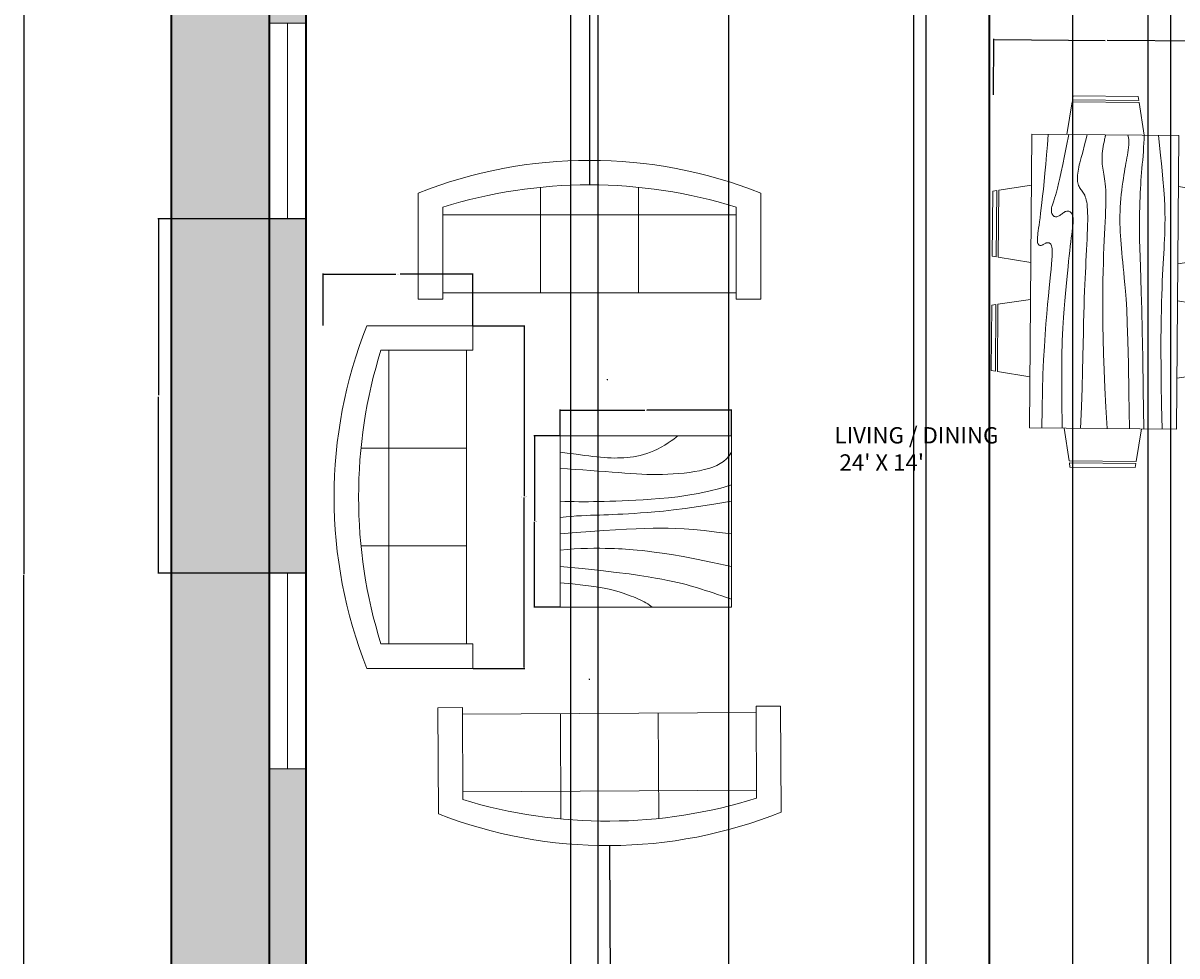
# Model space of a CAD drawing. Units: inches. Extents: x -7 to 546, y -27 to 766.
# Tile 5 of 9: x -7 to 276, y 276 to 505. Entities that reach past the tile are written whole.
import ezdxf

# ---------------------------------------------------------------- set-up
doc = ezdxf.new("R2010")
doc.units = ezdxf.units.IN
doc.header["$MEASUREMENT"] = 0
for name, color, linetype, lineweight in [('A-ANNO-DIMS', 2, 'Continuous', 18), ('A-AREA-IDEN', 7, 'Continuous', 18), ('A-WALL', 7, 'Continuous', 35), ('C-PROP', 7, 'Continuous', 35), ('furniture', 220, 'Continuous', 18), ('window', 30, 'Continuous', 20)]:
    doc.layers.add(name, color=color, linetype=linetype, lineweight=lineweight)
doc.layers.add('A-WALL-PATT', color=251, linetype='Continuous', lineweight=13, true_color=0x636466)
doc.layers.add('L-PLNT-PATT', color=85, linetype='Continuous', lineweight=13, true_color=0x58ba48)
doc.styles.get("Standard").update_dxf_attribs({"font": 'arial.ttf'})
doc.dimstyles.get("Standard").update_dxf_attribs({"dimtxt": 0.18, "dimasz": 0.18, "dimexe": 0.18, "dimexo": 0.0625, "dimgap": 0.09, "dimtad": 0, "dimtih": 1, "dimtoh": 1, "dimdec": 4, "dimzin": 0, "dimdsep": 46, "dimtxsty": 'Standard', "dimcen": 0.09, "dimadec": 0, "dimazin": 0, "dimtfac": 1, "dimtdec": 4, "dimtofl": 0, "dimtmove": 0, "dimatfit": 3, "dimfxl": 1, "dimtolj": 1, "dimtzin": 0, "dimarcsym": 0})

# ---------------------------------------------------------------- blocks, each defined once
blk = doc.blocks.new('Dining Set - 36 x 72 in.')
for p, q in [((-22.2343, 26.00059), (-23.4847, 17.99762)), ((-22.2304, 26), (-5.7608, 26)), ((-22, 27.5), (-22.1562, 26.50042)), ((-5.8416, 26.5), (-22.1534, 26.5)), ((-22, 27.5), (-6, 27.5)), ((-5.8437, 26.49966), (-6, 27.5)), ((-4.5152, 17.99762), (-5.7655, 25.99926)), ((5.7657, 26.00059), (4.5153, 17.99762)), ((5.7696, 26), (22.2392, 26)), ((6, 27.5), (5.8438, 26.50042)), ((22.1584, 26.5), (5.8466, 26.5)), ((6, 27.5), (22, 27.5)), ((22.1563, 26.49966), (22, 27.5)), ((23.4848, 17.99762), (22.2345, 25.99926)), ((36, 18), (-36, 18)), ((-36, 18), (-36, -18)), ((36, -18), (36, 18)), ((-44.0006, 8.23428), (-35.9976, 9.48474)), ((44.0006, 8.23428), (35.9976, 9.48474)), ((-45.5, 8), (-44.5004, 8.15617)), ((-45.5, 8), (-45.5, -8)), ((-44.5, -8.15843), (-44.5, 8.15338)), ((-44, 8.23041), (-44, -8.23915)), ((44, 8.23041), (44, -8.23915)), ((44.5, -8.15843), (44.5, 8.15338)), ((45.5, 8), (44.5005, 8.15617)), ((45.5, 8), (45.5, -8)), ((-44.4997, -8.15631), (-45.5, -8)), ((-35.9976, -9.48476), (-43.9993, -8.2345)), ((35.9976, -9.48476), (43.9993, -8.2345)), ((44.4997, -8.15631), (45.5, -8)), ((-36, -18), (36, -18)), ((-22.2343, -26.0006), (-23.4847, -17.99762)), ((-4.5152, -17.99762), (-5.7655, -25.99928)), ((5.7657, -26.0006), (4.5153, -17.99762)), ((23.4848, -17.99762), (22.2345, -25.99928)), ((-22.2304, -26), (-5.7608, -26)), ((-22, -27.5), (-22.1562, -26.50044)), ((-5.8416, -26.5), (-22.1534, -26.5)), ((-22, -27.5), (-6, -27.5)), ((-5.8437, -26.49967), (-6, -27.5)), ((5.7696, -26), (22.2392, -26)), ((6, -27.5), (5.8438, -26.50044)), ((22.1584, -26.5), (5.8466, -26.5)), ((6, -27.5), (22, -27.5)), ((22.1563, -26.49967), (22, -27.5))]:
    blk.add_line(p, q)
for points in [[(-36, 15), (-31.1772, 14.97754), (-26.8079, 14.91406), (-22.8538, 14.81543), (-19.276, 14.6875), (-16.0362, 14.53613), (-13.0957, 14.36718), (-10.4159, 14.18652), (-7.9583, 14), (-5.6904, 13.81315), (-3.6035, 13.63021), (-1.6954, 13.45508), (0.0365, 13.29166), (1.5945, 13.14388), (2.9811, 13.01562), (4.1988, 12.9108), (5.25, 12.83333), (6.1393, 12.78613), (6.8802, 12.76823), (7.4883, 12.77767), (7.9792, 12.8125), (8.3685, 12.87077), (8.6719, 12.95052), (8.9049, 13.0498), (9.0833, 13.16666), (9.2205, 13.29899), (9.3216, 13.44401), (9.3895, 13.59879), (9.4271, 13.76041), (9.4373, 13.92594), (9.4232, 14.09245), (9.3875, 14.257), (9.3333, 14.41666), (9.2638, 14.56917), (9.1836, 14.71484), (9.0975, 14.85465), (9.0104, 14.98958), (8.9272, 15.1206), (8.8529, 15.2487), (8.7922, 15.37483), (8.75, 15.5), (8.7305, 15.62467), (8.7344, 15.74739), (8.7617, 15.86621), (8.8125, 15.97916), (8.8867, 16.08431), (8.9844, 16.17968), (9.1055, 16.26334), (9.25, 16.33333), (9.4189, 16.38802), (9.6172, 16.42708), (9.8506, 16.45052), (10.125, 16.45833), (10.4463, 16.45052), (10.8203, 16.42708), (11.2529, 16.38802), (11.75, 16.33333), (12.3184, 16.26318), (12.9694, 16.17838), (13.7151, 16.07991), (14.5677, 15.96875), (15.5395, 15.84586), (16.6426, 15.71224), (17.8893, 15.56884), (19.2917, 15.41666), (20.859, 15.25667), (22.5879, 15.08984), (24.4721, 14.91715), (26.5052, 14.73958), (28.6809, 14.5581), (30.9929, 14.3737), (33.4347, 14.18733), (36, 14)], [(-36, 10), (-28.9766, 10.14274), (-23.1725, 10.20442), (-18.4241, 10.19775), (-14.5677, 10.13541), (-11.4399, 10.03011), (-8.877, 9.89453), (-6.7154, 9.74137), (-4.7917, 9.58333), (-2.9698, 9.43082), (-1.2246, 9.28515), (0.4415, 9.14534), (2.026, 9.01041), (3.5266, 8.87939), (4.9408, 8.7513), (6.266, 8.62516), (7.5, 8.5), (8.6411, 8.37549), (9.6914, 8.2539), (10.6538, 8.13818), (11.5312, 8.03125), (12.3267, 7.93603), (13.043, 7.85547), (13.6831, 7.79248), (14.25, 7.75), (14.7471, 7.7303), (15.1797, 7.73307), (15.5537, 7.75732), (15.875, 7.80208), (16.1494, 7.86637), (16.3828, 7.94922), (16.5811, 8.04964), (16.75, 8.16666), (16.8944, 8.29915), (17.0143, 8.44531), (17.1089, 8.60319), (17.1771, 8.77083), (17.218, 8.94629), (17.2305, 9.1276), (17.2137, 9.31282), (17.1667, 9.5), (17.0895, 9.6875), (16.987, 9.875), (16.8649, 10.0625), (16.7292, 10.25), (16.5856, 10.4375), (16.4401, 10.625), (16.2985, 10.8125), (16.1667, 11), (16.05, 11.18733), (15.9518, 11.3737), (15.8752, 11.5581), (15.8229, 11.73958), (15.798, 11.91715), (15.8034, 12.08984), (15.842, 12.25667), (15.9167, 12.41666), (16.0295, 12.56836), (16.1784, 12.70833), (16.3605, 12.83268), (16.5729, 12.9375), (16.8127, 13.01888), (17.0768, 13.07291), (17.3625, 13.0957), (17.6667, 13.08333), (17.9894, 13.03312), (18.3418, 12.94726), (18.7382, 12.82918), (19.1927, 12.68229), (19.7195, 12.51001), (20.3327, 12.31575), (21.0465, 12.10294), (21.875, 11.875), (22.8357, 11.63354), (23.959, 11.37304), (25.2786, 11.08618), (26.8282, 10.76562), (28.6414, 10.40405), (30.752, 9.99414), (33.1936, 9.52856), (36, 9)], [(-36, 5.5), (-30.7157, 5.3348), (-26.069, 5.20963), (-21.9946, 5.11767), (-18.4271, 5.05208), (-15.3009, 5.00602), (-12.5508, 4.97265), (-10.1112, 4.94515), (-7.9167, 4.91666), (-5.909, 4.88167), (-4.0586, 4.83984), (-2.3429, 4.79215), (-0.7396, 4.73958), (0.7739, 4.6831), (2.22, 4.6237), (3.6213, 4.56233), (5, 4.5), (6.373, 4.43782), (7.7344, 4.3776), (9.0723, 4.32129), (10.375, 4.27083), (11.6309, 4.22819), (12.8281, 4.19531), (13.9551, 4.17415), (15, 4.16666), (15.954, 4.17448), (16.819, 4.19791), (17.6001, 4.23698), (18.3021, 4.29166), (18.9299, 4.36198), (19.4883, 4.44791), (19.9823, 4.54948), (20.4167, 4.66666), (20.7969, 4.79899), (21.1302, 4.94401), (21.4245, 5.09879), (21.6875, 5.26041), (21.9271, 5.42594), (22.1511, 5.59245), (22.3672, 5.757), (22.5834, 5.91666), (22.8065, 6.06868), (23.0404, 6.21093), (23.2879, 6.34147), (23.5521, 6.45833), (23.8358, 6.55957), (24.142, 6.64323), (24.4735, 6.70735), (24.8334, 6.75), (25.2235, 6.76969), (25.642, 6.76692), (26.0858, 6.74267), (26.5521, 6.69791), (27.0379, 6.63362), (27.5404, 6.55078), (28.0565, 6.45036), (28.5834, 6.33333), (29.1242, 6.19987), (29.7071, 6.04687), (30.3661, 5.87044), (31.1354, 5.66666), (32.0493, 5.43164), (33.142, 5.16146), (34.4475, 4.85221), (36, 4.5)], [(-36, -1), (-30.7915, -0.6591), (-26.0195, -0.38216), (-21.6519, -0.16284), (-17.6563, 0.00521), (-14.0005, 0.12833), (-10.6523, 0.21289), (-7.5796, 0.26522), (-4.75, 0.29166), (-2.134, 0.29793), (0.2878, 0.28711), (2.5317, 0.26163), (4.6146, 0.22396), (6.5529, 0.17651), (8.3633, 0.12174), (10.0623, 0.06209), (11.6667, 0), (13.1899, -0.06201), (14.6341, -0.1211), (15.9982, -0.17432), (17.2813, -0.21875), (18.4823, -0.25147), (19.6003, -0.26953), (20.6343, -0.27002), (21.5834, -0.25), (22.4481, -0.20768), (23.2357, -0.14584), (23.9549, -0.06836), (24.6146, 0.02083), (25.2235, 0.11784), (25.7904, 0.21875), (26.3241, 0.31966), (26.8334, 0.41666), (27.3265, 0.50618), (27.8099, 0.58593), (28.2894, 0.65397), (28.7709, 0.70833), (29.2601, 0.74707), (29.763, 0.76823), (30.2855, 0.76985), (30.8334, 0.75), (31.4088, 0.70784), (31.9994, 0.64713), (32.589, 0.57275), (33.1615, 0.48958), (33.7008, 0.4025), (34.1908, 0.3164), (34.6153, 0.23616), (34.9584, 0.16666), (35.2099, 0.11165), (35.3848, 0.07031), (35.504, 0.04069), (35.5886, 0.02083), (35.6594, 0.00879), (35.7377, 0.0026), (35.8442, 0.00032), (36, 0)], [(-36, -6.5), (-27.1843, -6.31267), (-20.084, -6.1263), (-14.469, -5.9419), (-10.1094, -5.76042), (-6.7752, -5.58285), (-4.2363, -5.41016), (-2.2629, -5.24333), (-0.625, -5.08334), (0.8708, -4.93099), (2.2715, -4.78646), (3.5872, -4.64974), (4.8281, -4.52084), (6.0046, -4.39974), (7.127, -4.28646), (8.2053, -4.18099), (9.25, -4.08334), (10.2705, -3.99382), (11.2734, -3.91407), (12.2647, -3.84603), (13.25, -3.79167), (14.2354, -3.75293), (15.2266, -3.73177), (16.2295, -3.73015), (17.25, -3.75), (18.2912, -3.79248), (19.3451, -3.85547), (20.4009, -3.93604), (21.4479, -4.03125), (22.4754, -4.13819), (23.4727, -4.25391), (24.4289, -4.37549), (25.3334, -4.5), (26.1785, -4.62492), (26.9694, -4.74935), (27.7145, -4.87281), (28.4219, -4.99479), (29.1, -5.11483), (29.7572, -5.23242), (30.4016, -5.34709), (31.0417, -5.45834), (31.6837, -5.56437), (32.3262, -5.65821), (32.9658, -5.73153), (33.599, -5.77604), (34.2224, -5.78345), (34.8327, -5.74545), (35.4264, -5.65373), (36, -5.5)], [(-36, -10), (-26.4022, -9.81299), (-18.4675, -9.62891), (-11.9839, -9.45069), (-6.7396, -9.28125), (-2.5226, -9.12354), (0.8789, -8.98047), (3.6769, -8.85498), (6.0833, -8.75), (8.2767, -8.66765), (10.3021, -8.60677), (12.1712, -8.56543), (13.8958, -8.54167), (15.4876, -8.53353), (16.9583, -8.53907), (18.3197, -8.55632), (19.5834, -8.58334), (20.7616, -8.61841), (21.8685, -8.66081), (22.9188, -8.71004), (23.9271, -8.76563), (24.9081, -8.82707), (25.8763, -8.89388), (26.8465, -8.96558), (27.8334, -9.04167), (28.8474, -9.12118), (29.8828, -9.20117), (30.93, -9.27824), (31.9792, -9.34896), (33.0205, -9.40991), (34.0443, -9.45768), (35.0407, -9.48885), (36, -9.5)], [(-36, -14.5), (-30.0881, -14.33513), (-25.0332, -14.21224), (-20.7312, -14.12647), (-17.0781, -14.07292), (-13.97, -14.04671), (-11.3027, -14.04297), (-8.9724, -14.05681), (-6.875, -14.08334), (-4.9224, -14.11833), (-3.0905, -14.16016), (-1.3709, -14.20785), (0.2448, -14.26042), (1.7647, -14.3169), (3.1973, -14.3763), (4.5507, -14.43767), (5.8333, -14.5), (7.0554, -14.5621), (8.235, -14.62175), (9.3922, -14.67652), (10.5469, -14.72396), (11.7192, -14.76164), (12.929, -14.78711), (14.1965, -14.79794), (15.5417, -14.79167), (16.9933, -14.76424), (18.6152, -14.70508), (20.4804, -14.60197), (22.6615, -14.44271), (25.2312, -14.21509), (28.2624, -13.9069), (31.8277, -13.50594), (36, -13)]]:
    blk.add_lwpolyline(points)
blk = doc.blocks.new('Sofa - Roundback 7 ft.')
for p, q in [((-12.00002, -32.4421), (-12.00003, -6.5971)), ((11.99997, -32.4421), (11.99998, -6.5971)), ((-36.000027, -34), (-36.000027, -11.4696)), ((-35.999844, -13.3819), (35.9998, -13.3819)), ((35.99998, -34), (35.99998, -11.4696)), ((-36.000027, -32.4421), (35.99998, -32.4421))]:
    blk.add_line(p, q)
for points in [[(-36.000027, -34), (-42.000027, -34), (-42.000027, -8)], [(41.99998, -8), (41.99998, -34), (35.99998, -34)]]:
    blk.add_lwpolyline(points)
for centre, radius, start, end in [((0, -114.25), 114.25, 68.43141, 111.5686), ((-0.00001, -127.1968), 121.1968, 72.72033, 107.2797)]:
    blk.add_arc(centre, radius, start, end)
blk = doc.blocks.new('Table - Square Woodgrain 42 x 42 in.')
blk.add_line((0, -42), (42, -42))
for points in [[(0, -4), (1.704, -4.2172), (3.2358, -4.4188), (4.615, -4.604), (5.8615, -4.7721), (6.9951, -4.9224), (8.0357, -5.0541), (9.0031, -5.1667), (9.9171, -5.2594), (10.7951, -5.3316), (11.6445, -5.3836), (12.4702, -5.4157), (13.277, -5.4283), (14.0698, -5.4217), (14.8535, -5.3964), (15.6331, -5.3526), (16.4133, -5.2908), (17.1986, -5.2103), (17.9913, -5.1062), (18.793, -4.9727), (19.6056, -4.8038), (20.4307, -4.5937), (21.2701, -4.3365), (22.1256, -4.0262), (22.9989, -3.6571), (23.888, -3.2272), (24.7756, -2.7516), (25.6408, -2.2491), (26.4624, -1.7387), (27.2195, -1.2395), (27.891, -0.7703), (28.456, -0.3501), (28.8934, 0.002)], [(0, -42), (0, 0), (42, 0), (42, -42)], [(0, -8), (1.8203, -8.1001), (3.6741, -8.2149), (5.5411, -8.3408), (7.4011, -8.4741), (9.2339, -8.6112), (11.0193, -8.7484), (12.7371, -8.8821), (14.3671, -9.0086), (15.8954, -9.1246), (17.3337, -9.2278), (18.6997, -9.3159), (20.0116, -9.387), (21.2871, -9.4389), (22.5442, -9.4696), (23.8008, -9.477), (25.0749, -9.459), (26.3791, -9.4137), (27.7049, -9.3403), (29.0383, -9.2382), (30.3655, -9.1068), (31.6728, -8.9455), (32.9461, -8.7535), (34.1717, -8.5304), (35.3358, -8.2756), (36.4268, -7.9863), (37.443, -7.6521), (38.3849, -7.2603), (39.253, -6.7986), (40.048, -6.2542), (40.7705, -5.6147), (41.421, -4.8674), (42, -4)], [(42, -12), (39.1784, -12.8621), (36.4519, -13.5654), (33.8246, -14.1294), (31.3004, -14.5731), (28.8832, -14.9161), (26.577, -15.1775), (24.3858, -15.3768), (22.3136, -15.5332), (20.3622, -15.6632), (18.5254, -15.7718), (16.7947, -15.8612), (15.1618, -15.9338), (13.6183, -15.9916), (12.1558, -16.0369), (10.7659, -16.0718), (9.4403, -16.0987), (8.1703, -16.1191), (6.9461, -16.1325), (5.7577, -16.1377), (4.595, -16.1335), (3.4479, -16.1188), (2.3064, -16.0924), (1.1604, -16.0532), (0, -16)], [(42, -16), (37.6529, -16.7365), (33.8802, -17.329), (30.6179, -17.7961), (27.8015, -18.1561), (25.3668, -18.4275), (23.2497, -18.6288), (21.3859, -18.7785), (19.7111, -18.8949), (18.1693, -18.9939), (16.7375, -19.0795), (15.401, -19.1534), (14.1449, -19.217), (12.9544, -19.2717), (11.8148, -19.3191), (10.7113, -19.3606), (9.6291, -19.3976), (8.5534, -19.4323), (7.47, -19.4689), (6.3643, -19.5122), (5.222, -19.5672), (4.0288, -19.6386), (2.7703, -19.7313), (1.4321, -19.8501), (0, -20)], [(0, -24), (3.9243, -23.6805), (7.4766, -23.4138), (10.6891, -23.1954), (13.5943, -23.0205), (16.2247, -22.8847), (18.6125, -22.7832), (20.7903, -22.7116), (22.7903, -22.6651), (24.6563, -22.642), (26.4764, -22.6507), (28.35, -22.7024), (30.3766, -22.8084), (32.6555, -22.98), (35.2861, -23.2283), (38.3678, -23.5645), (42, -24)], [(42, -32), (37.392, -31.017), (33.4585, -30.2231), (30.1291, -29.5949), (27.3334, -29.109), (25.0009, -28.742), (23.0612, -28.4707), (21.4439, -28.2716), (20.0786, -28.1215), (18.8998, -28.0002), (17.8609, -27.9014), (16.9206, -27.8219), (16.0371, -27.7588), (15.1691, -27.709), (14.2748, -27.6693), (13.3128, -27.6368), (12.2415, -27.6083), (11.0295, -27.5824), (9.6867, -27.5643), (8.233, -27.5608), (6.6884, -27.5787), (5.0728, -27.6248), (3.4062, -27.7058), (1.7086, -27.8286), (0, -28)], [(0, -32), (5.4026, -32.5358), (9.9494, -33.019), (13.7424, -33.4553), (16.8834, -33.8505), (19.4743, -34.2106), (21.6171, -34.5413), (23.4136, -34.8486), (24.9657, -35.1382), (26.3614, -35.4156), (27.6332, -35.6841), (28.7995, -35.9467), (29.8788, -36.2064), (30.8897, -36.4661), (31.8507, -36.7288), (32.7802, -36.9973), (33.6968, -37.2747), (34.6175, -37.5635), (35.5531, -37.8651), (36.5128, -38.1805), (37.506, -38.5108), (38.5421, -38.8568), (39.6302, -39.2197), (40.7797, -39.6004), (42, -40)], [(0, -36), (3.0098, -36.2857), (5.5354, -36.5643), (7.6368, -36.8359), (9.374, -37.1009), (10.807, -37.3597), (11.9957, -37.6126), (13.0002, -37.8599), (13.8804, -38.102), (14.6874, -38.3393), (15.4365, -38.5729), (16.1338, -38.8041), (16.7858, -39.0341), (17.3987, -39.264), (17.9787, -39.4952), (18.5322, -39.7288), (19.0655, -39.9662), (19.5832, -40.2081), (20.0842, -40.4544), (20.5657, -40.7046), (21.0249, -40.9581), (21.459, -41.2144), (21.8653, -41.4731), (22.2409, -41.7335), (22.5831, -41.9951)]]:
    blk.add_lwpolyline(points)
blk = doc.blocks.new('WIN-48IN')
for p, q in [((0, 9), (0, 0)), ((48, 9), (0, 9)), ((0, 9), (0, 4.5)), ((48, 0), (48, 9)), ((0, 4.5), (48, 4.5)), ((0, 0), (48, 0))]:
    blk.add_line(p, q)
blk = doc.blocks.new('*D20')
at = {"layer": 'A-ANNO-DIMS', "color": 0, "lineweight": -2, "transparency": 16777216}
for p, q in [((103.24, 430.74), (115.95, 430.74)), ((115.77, 430.56), (115.77, 388.92)), ((115.77, 346.92), (115.77, 388.56)), ((103.24, 346.74), (115.95, 346.74))]:
    blk.add_line(p, q, dxfattribs=at)
at = {"layer": 'A-ANNO-DIMS', "color": 0, "transparency": 16777216}
for points in [[(115.74, 430.56), (115.8, 430.56), (115.77, 430.74)], [(115.74, 346.92), (115.8, 346.92), (115.77, 346.74)]]:
    blk.add_solid(points, dxfattribs=at)
at = {"layer": 'Defpoints', "color": 0, "transparency": 16777216}
for p in [(103.17, 430.74), (115.77, 430.74), (103.17, 346.74)]:
    blk.add_point(p, dxfattribs=at)
at = {"layer": 'A-ANNO-DIMS', "color": 0, "transparency": 16777216, "insert": (115.77, 388.74), "char_height": 0.18, "attachment_point": 5}
blk.add_mtext('\\A1;SOFA 84 TYP.', dxfattribs=at)
blk = doc.blocks.new('*D21')
at = {"layer": 'A-ANNO-DIMS', "color": 0, "lineweight": -2, "transparency": 16777216}
for p, q in [((66.51, 430.8), (66.51, 443.52)), ((66.69, 443.34), (84.31, 443.34)), ((102.99, 443.34), (85.37, 443.34)), ((103.17, 430.8), (103.17, 443.52))]:
    blk.add_line(p, q, dxfattribs=at)
at = {"layer": 'A-ANNO-DIMS', "color": 0, "transparency": 16777216}
for points in [[(66.69, 443.37), (66.69, 443.31), (66.51, 443.34)], [(102.99, 443.37), (102.99, 443.31), (103.17, 443.34)]]:
    blk.add_solid(points, dxfattribs=at)
at = {"layer": 'Defpoints', "color": 0, "transparency": 16777216}
for p in [(66.51, 443.34), (66.51, 430.74), (103.17, 430.74)]:
    blk.add_point(p, dxfattribs=at)
at = {"layer": 'A-ANNO-DIMS', "color": 0, "transparency": 16777216, "insert": (84.84, 443.34), "char_height": 0.18, "attachment_point": 5}
blk.add_mtext('\\A1;37 TYP.', dxfattribs=at)
blk = doc.blocks.new('*D25')
at = {"layer": 'A-ANNO-DIMS', "color": 0, "lineweight": -2, "transparency": 16777216}
for p, q in [((230.87, 487.32), (230.98, 501.09)), ((231.16, 500.91), (258.26, 500.68)), ((285.8, 500.45), (258.7, 500.68)), ((285.87, 486.86), (285.98, 500.63))]:
    blk.add_line(p, q, dxfattribs=at)
at = {"layer": 'A-ANNO-DIMS', "color": 0, "transparency": 16777216}
for points in [[(231.16, 500.94), (231.16, 500.88), (230.98, 500.91)], [(285.8, 500.48), (285.8, 500.42), (285.98, 500.45)]]:
    blk.add_solid(points, dxfattribs=at)
at = {"layer": 'Defpoints', "color": 0, "transparency": 16777216}
for p in [(230.98, 500.91), (230.87, 487.26), (285.87, 486.8)]:
    blk.add_point(p, dxfattribs=at)
at = {"layer": 'A-ANNO-DIMS', "color": 0, "transparency": 16777216, "insert": (258.48, 500.68), "char_height": 0.18, "attachment_point": 5}
blk.add_mtext('\\A1;55', dxfattribs=at)
blk = doc.blocks.new('*D26')
at = {"layer": 'A-ANNO-DIMS', "color": 0, "lineweight": -2, "transparency": 16777216}
for p, q in [((124.54, 403.73), (118.12, 403.73)), ((118.3, 403.55), (118.3, 382.91)), ((118.3, 361.91), (118.3, 382.55)), ((124.54, 361.73), (118.12, 361.73))]:
    blk.add_line(p, q, dxfattribs=at)
at = {"layer": 'A-ANNO-DIMS', "color": 0, "transparency": 16777216}
for points in [[(118.27, 403.55), (118.33, 403.55), (118.3, 403.73)], [(118.27, 361.91), (118.33, 361.91), (118.3, 361.73)]]:
    blk.add_solid(points, dxfattribs=at)
at = {"layer": 'Defpoints', "color": 0, "transparency": 16777216}
for p in [(118.3, 403.73), (124.6, 403.73), (124.6, 361.73)]:
    blk.add_point(p, dxfattribs=at)
at = {"layer": 'A-ANNO-DIMS', "color": 0, "transparency": 16777216, "insert": (118.3, 382.73), "char_height": 0.18, "attachment_point": 5}
blk.add_mtext('\\A1;TABLE 42', dxfattribs=at)
blk = doc.blocks.new('*D27')
at = {"layer": 'A-ANNO-DIMS', "color": 0, "lineweight": -2, "transparency": 16777216}
for p, q in [((124.6, 403.8), (124.6, 410.21)), ((124.78, 410.03), (145.38, 410.03)), ((166.42, 410.03), (145.82, 410.03)), ((166.6, 403.8), (166.6, 410.21))]:
    blk.add_line(p, q, dxfattribs=at)
at = {"layer": 'A-ANNO-DIMS', "color": 0, "transparency": 16777216}
for points in [[(124.78, 410.06), (124.78, 410), (124.6, 410.03)], [(166.42, 410.06), (166.42, 410), (166.6, 410.03)]]:
    blk.add_solid(points, dxfattribs=at)
at = {"layer": 'Defpoints', "color": 0, "transparency": 16777216}
for p in [(166.6, 410.03), (124.6, 403.73), (166.6, 403.73)]:
    blk.add_point(p, dxfattribs=at)
at = {"layer": 'A-ANNO-DIMS', "color": 0, "transparency": 16777216, "insert": (145.6, 410.03), "char_height": 0.18, "attachment_point": 5}
blk.add_mtext('\\A1;42', dxfattribs=at)
blk = doc.blocks.new('*D31')
at = {"layer": 'A-ANNO-DIMS', "color": 0, "lineweight": -2, "transparency": 16777216}
for p, q in [((29.17, 729.74), (-7.07, 729.74)), ((-6.89, 729.56), (-6.89, 369.93)), ((-6.89, 9.92), (-6.89, 369.56)), ((29.17, 9.74), (-7.07, 9.74))]:
    blk.add_line(p, q, dxfattribs=at)
at = {"layer": 'A-ANNO-DIMS', "color": 0, "transparency": 16777216}
for points in [[(-6.92, 729.56), (-6.86, 729.56), (-6.89, 729.74)], [(-6.92, 9.92), (-6.86, 9.92), (-6.89, 9.74)]]:
    blk.add_solid(points, dxfattribs=at)
at = {"layer": 'Defpoints', "color": 0, "transparency": 16777216}
for p in [(-6.89, 729.74), (29.23, 729.74), (29.23, 9.74)]:
    blk.add_point(p, dxfattribs=at)
at = {"layer": 'A-ANNO-DIMS', "color": 0, "transparency": 16777216, "insert": (-6.89, 369.74), "char_height": 0.18, "attachment_point": 5}
blk.add_mtext('\\A1;720', dxfattribs=at)
blk = doc.blocks.new('*D39')
at = {"layer": 'A-ANNO-DIMS', "color": 0, "lineweight": -2, "transparency": 16777216}
for p, q in [((214.23, 600.68), (214.23, -26.56)), ((250.23, 600.68), (250.23, -26.56)), ((214.41, -26.38), (232.01, -26.38)), ((250.05, -26.38), (232.45, -26.38))]:
    blk.add_line(p, q, dxfattribs=at)
at = {"layer": 'A-ANNO-DIMS', "color": 0, "transparency": 16777216}
for points in [[(214.41, -26.35), (214.41, -26.41), (214.23, -26.38)], [(250.05, -26.35), (250.05, -26.41), (250.23, -26.38)]]:
    blk.add_solid(points, dxfattribs=at)
at = {"layer": 'Defpoints', "color": 0, "transparency": 16777216}
for p in [(214.23, 600.74), (250.23, 600.74), (250.23, -26.38)]:
    blk.add_point(p, dxfattribs=at)
at = {"layer": 'A-ANNO-DIMS', "color": 0, "transparency": 16777216, "insert": (232.23, -26.38), "char_height": 0.18, "attachment_point": 5}
blk.add_mtext('\\A1;36', dxfattribs=at)
blk = doc.blocks.new('*D41')
at = {"layer": 'A-ANNO-DIMS', "color": 0, "lineweight": -2, "transparency": 16777216}
for p, q in [((274.23, 600.68), (274.23, -26.56)), ((279.23, 600.68), (279.23, -26.56)), ((274.41, -26.38), (276.58, -26.38)), ((279.05, -26.38), (276.88, -26.38))]:
    blk.add_line(p, q, dxfattribs=at)
at = {"layer": 'A-ANNO-DIMS', "color": 0, "transparency": 16777216}
for points in [[(274.41, -26.35), (274.41, -26.41), (274.23, -26.38)], [(279.05, -26.35), (279.05, -26.41), (279.23, -26.38)]]:
    blk.add_solid(points, dxfattribs=at)
at = {"layer": 'Defpoints', "color": 0, "transparency": 16777216}
for p in [(274.23, 600.74), (279.23, 600.74), (279.23, -26.38)]:
    blk.add_point(p, dxfattribs=at)
at = {"layer": 'A-ANNO-DIMS', "color": 0, "transparency": 16777216, "insert": (276.73, -26.38), "char_height": 0.18, "attachment_point": 5}
blk.add_mtext('\\A1;5', dxfattribs=at)
blk = doc.blocks.new('*D42')
at = {"layer": 'A-ANNO-DIMS', "color": 0, "lineweight": -2, "transparency": 16777216}
for p, q in [((211.23, 696.68), (211.23, -26.56)), ((229.74, 696.68), (229.74, -26.56)), ((211.41, -26.38), (220.12, -26.38)), ((229.56, -26.38), (220.85, -26.38))]:
    blk.add_line(p, q, dxfattribs=at)
at = {"layer": 'A-ANNO-DIMS', "color": 0, "transparency": 16777216}
for points in [[(211.41, -26.35), (211.41, -26.41), (211.23, -26.38)], [(229.56, -26.35), (229.56, -26.41), (229.74, -26.38)]]:
    blk.add_solid(points, dxfattribs=at)
at = {"layer": 'Defpoints', "color": 0, "transparency": 16777216}
for p in [(211.23, 696.74), (229.74, 696.74), (229.74, -26.38)]:
    blk.add_point(p, dxfattribs=at)
at = {"layer": 'A-ANNO-DIMS', "color": 0, "transparency": 16777216, "insert": (220.49, -26.38), "char_height": 0.18, "attachment_point": 5}
blk.add_mtext('\\A1;18.51', dxfattribs=at)
blk = doc.blocks.new('*D45')
at = {"layer": 'A-ANNO-DIMS', "color": 0, "lineweight": -2, "transparency": 16777216}
for p, q in [((211.23, 600.68), (211.23, -26.56)), ((214.23, 600.68), (214.23, -26.56)), ((211.41, -26.38), (212.58, -26.38)), ((214.05, -26.38), (212.88, -26.38))]:
    blk.add_line(p, q, dxfattribs=at)
at = {"layer": 'A-ANNO-DIMS', "color": 0, "transparency": 16777216}
for points in [[(211.41, -26.35), (211.41, -26.41), (211.23, -26.38)], [(214.05, -26.35), (214.05, -26.41), (214.23, -26.38)]]:
    blk.add_solid(points, dxfattribs=at)
at = {"layer": 'Defpoints', "color": 0, "transparency": 16777216}
for p in [(211.23, 600.74), (214.23, 600.74), (214.23, -26.38)]:
    blk.add_point(p, dxfattribs=at)
at = {"layer": 'A-ANNO-DIMS', "color": 0, "transparency": 16777216, "insert": (212.73, -26.38), "char_height": 0.18, "attachment_point": 5}
blk.add_mtext('\\A1;3', dxfattribs=at)
blk = doc.blocks.new('*D53')
at = {"layer": 'A-ANNO-DIMS', "color": 0, "lineweight": -2, "transparency": 16777216}
for p, q in [((133.93, 124.01), (133.93, 766.05)), ((134.11, 765.87), (181.71, 765.87)), ((229.75, 765.87), (182.15, 765.87)), ((229.93, 124.01), (229.93, 766.05))]:
    blk.add_line(p, q, dxfattribs=at)
at = {"layer": 'A-ANNO-DIMS', "color": 0, "transparency": 16777216}
for points in [[(134.11, 765.9), (134.11, 765.84), (133.93, 765.87)], [(229.75, 765.9), (229.75, 765.84), (229.93, 765.87)]]:
    blk.add_solid(points, dxfattribs=at)
at = {"layer": 'Defpoints', "color": 0, "transparency": 16777216}
for p in [(229.93, 765.87), (133.93, 123.94), (229.93, 123.94)]:
    blk.add_point(p, dxfattribs=at)
at = {"layer": 'A-ANNO-DIMS', "color": 0, "transparency": 16777216, "insert": (181.93, 765.87), "char_height": 0.18, "attachment_point": 5}
blk.add_mtext('\\A1;96', dxfattribs=at)
blk = doc.blocks.new('*D68')
at = {"layer": 'A-ANNO-DIMS', "color": 0, "lineweight": -2, "transparency": 16777216}
for p, q in [((133.93, 100.01), (133.93, 766.05)), ((134.11, 765.87), (149.71, 765.87)), ((165.75, 765.87), (150.15, 765.87)), ((165.93, 104.01), (165.93, 766.05))]:
    blk.add_line(p, q, dxfattribs=at)
at = {"layer": 'A-ANNO-DIMS', "color": 0, "transparency": 16777216}
for points in [[(134.11, 765.9), (134.11, 765.84), (133.93, 765.87)], [(165.75, 765.9), (165.75, 765.84), (165.93, 765.87)]]:
    blk.add_solid(points, dxfattribs=at)
at = {"layer": 'Defpoints', "color": 0, "transparency": 16777216}
for p in [(165.93, 765.87), (165.93, 103.94), (133.93, 99.94)]:
    blk.add_point(p, dxfattribs=at)
at = {"layer": 'A-ANNO-DIMS', "color": 0, "transparency": 16777216, "insert": (149.93, 765.87), "char_height": 0.18, "attachment_point": 5}
blk.add_mtext('\\A1;32', dxfattribs=at)
blk = doc.blocks.new('*D73')
at = {"layer": 'A-ANNO-DIMS', "color": 0, "lineweight": -2, "transparency": 16777216}
for p, q in [((62.16, 456.93), (25.92, 456.93)), ((26.1, 456.75), (26.1, 413.69)), ((26.1, 370.27), (26.1, 413.33)), ((62.16, 370.09), (25.92, 370.09))]:
    blk.add_line(p, q, dxfattribs=at)
at = {"layer": 'A-ANNO-DIMS', "color": 0, "transparency": 16777216}
for points in [[(26.07, 456.75), (26.13, 456.75), (26.1, 456.93)], [(26.07, 370.27), (26.13, 370.27), (26.1, 370.09)]]:
    blk.add_solid(points, dxfattribs=at)
at = {"layer": 'Defpoints', "color": 0, "transparency": 16777216}
for p in [(26.1, 456.93), (62.23, 456.93), (62.23, 370.09)]:
    blk.add_point(p, dxfattribs=at)
at = {"layer": 'A-ANNO-DIMS', "color": 0, "transparency": 16777216, "insert": (26.1, 413.51), "char_height": 0.18, "attachment_point": 5}
blk.add_mtext('\\A1;86.83', dxfattribs=at)
blk = doc.blocks.new('*D81')
at = {"layer": 'A-ANNO-DIMS', "color": 0, "lineweight": -2, "transparency": 16777216}
for p, q in [((62.23, 240.81), (62.23, 766.05)), ((62.41, 765.87), (194.44, 765.87)), ((327.05, 765.87), (195.02, 765.87)), ((327.23, 234.81), (327.23, 766.05))]:
    blk.add_line(p, q, dxfattribs=at)
at = {"layer": 'A-ANNO-DIMS', "color": 0, "transparency": 16777216}
for points in [[(62.41, 765.9), (62.41, 765.84), (62.23, 765.87)], [(327.05, 765.9), (327.05, 765.84), (327.23, 765.87)]]:
    blk.add_solid(points, dxfattribs=at)
at = {"layer": 'Defpoints', "color": 0, "transparency": 16777216}
for p in [(327.23, 765.87), (62.23, 240.74), (327.23, 234.74)]:
    blk.add_point(p, dxfattribs=at)
at = {"layer": 'A-ANNO-DIMS', "color": 0, "transparency": 16777216, "insert": (194.73, 765.87), "char_height": 0.18, "attachment_point": 5}
blk.add_mtext('\\A1;265', dxfattribs=at)
blk = doc.blocks.new('*D83')
at = {"layer": 'A-ANNO-DIMS', "color": 0, "lineweight": -2, "transparency": 16777216}
for p, q in [((127.23, 91.81), (127.23, 766.05)), ((127.41, 765.87), (130.18, 765.87)), ((133.75, 765.87), (130.97, 765.87)), ((133.93, 100.01), (133.93, 766.05))]:
    blk.add_line(p, q, dxfattribs=at)
at = {"layer": 'A-ANNO-DIMS', "color": 0, "transparency": 16777216}
for points in [[(127.41, 765.9), (127.41, 765.84), (127.23, 765.87)], [(133.75, 765.9), (133.75, 765.84), (133.93, 765.87)]]:
    blk.add_solid(points, dxfattribs=at)
at = {"layer": 'Defpoints', "color": 0, "transparency": 16777216}
for p in [(133.93, 765.87), (133.93, 99.94), (127.23, 91.74)]:
    blk.add_point(p, dxfattribs=at)
at = {"layer": 'A-ANNO-DIMS', "color": 0, "transparency": 16777216, "insert": (130.58, 765.87), "char_height": 0.18, "attachment_point": 5}
blk.add_mtext('\\A1;6.695', dxfattribs=at)
blk = doc.blocks.new('*D85')
at = {"layer": 'A-ANNO-DIMS', "color": 0, "lineweight": -2, "transparency": 16777216}
for p, q in [((274.23, 696.68), (274.23, -26.56)), ((268.74, 692.17), (268.74, -26.56)), ((268.92, -26.38), (271.09, -26.38)), ((274.05, -26.38), (271.88, -26.38))]:
    blk.add_line(p, q, dxfattribs=at)
at = {"layer": 'A-ANNO-DIMS', "color": 0, "transparency": 16777216}
for points in [[(268.92, -26.35), (268.92, -26.41), (268.74, -26.38)], [(274.05, -26.35), (274.05, -26.41), (274.23, -26.38)]]:
    blk.add_solid(points, dxfattribs=at)
at = {"layer": 'Defpoints', "color": 0, "transparency": 16777216}
for p in [(274.23, 696.74), (268.74, 692.23), (268.74, -26.38)]:
    blk.add_point(p, dxfattribs=at)
at = {"layer": 'A-ANNO-DIMS', "color": 0, "transparency": 16777216, "insert": (271.49, -26.38), "char_height": 0.18, "attachment_point": 5}
blk.add_mtext('\\A1;5.493', dxfattribs=at)
blk = doc.blocks.new('*D89')
at = {"layer": 'A-ANNO-DIMS', "color": 0, "lineweight": -2, "transparency": 16777216}
for p, q in [((131.97, 537.98), (131.79, 537.98)), ((131.79, 537.98), (131.79, 465.44)), ((131.7, 344.07), (131.88, 344.07)), ((131.79, 343.98), (131.79, 344.16))]:
    blk.add_line(p, q, dxfattribs=at)
at = {"layer": 'A-ANNO-DIMS', "color": 0, "transparency": 16777216}
blk.add_solid([(131.76, 465.44), (131.82, 465.44), (131.79, 465.26)], dxfattribs=at)
at = {"layer": 'Defpoints', "color": 0, "transparency": 16777216}
for p in [(131.79, 465.26), (131.79, 344.07)]:
    blk.add_point(p, dxfattribs=at)
at = {"layer": 'A-ANNO-DIMS', "color": 0, "transparency": 16777216, "insert": (132.65, 537.98), "char_height": 0.18, "attachment_point": 5}
blk.add_mtext('\\A1;3X R121.2', dxfattribs=at)
blk = doc.blocks.new('*D90')
at = {"layer": 'A-ANNO-DIMS', "color": 0, "lineweight": -2, "transparency": 16777216}
for p, q in [((136.15, 417.53), (136.33, 417.53)), ((136.24, 417.44), (136.24, 417.62)), ((137.16, 234.74), (136.81, 303.11)), ((137.34, 234.74), (137.16, 234.74))]:
    blk.add_line(p, q, dxfattribs=at)
at = {"layer": 'A-ANNO-DIMS', "color": 0, "transparency": 16777216}
blk.add_solid([(136.84, 303.11), (136.78, 303.11), (136.81, 303.29)], dxfattribs=at)
at = {"layer": 'Defpoints', "color": 0, "transparency": 16777216}
for p in [(136.24, 417.53), (136.81, 303.29)]:
    blk.add_point(p, dxfattribs=at)
at = {"layer": 'A-ANNO-DIMS', "color": 0, "transparency": 16777216, "insert": (138.08, 234.74), "char_height": 0.18, "attachment_point": 5}
blk.add_mtext('\\A1;3X R114.25', dxfattribs=at)

msp = doc.modelspace()

# ---------------------------------------------------------------- hatches: boundary and pattern name
at = {"layer": 'A-WALL-PATT'}
h = msp.add_hatch(color=256, dxfattribs=at)
h.dxf.hatch_style = 1
h.paths.add_polyline_path([(62.2319, 696.744), (86.6896, 696.744), (86.6896, 705.744), (53.2319, 705.744), (53.2319, 627.8642), (57.7271, 627.8642), (62.2319, 627.8642)])
h.paths.add_polyline_path([(229.7414, 705.744), (134.6896, 705.744), (134.6896, 696.744), (206.2319, 696.744), (206.2319, 567.744), (211.2319, 567.744), (211.2319, 595.744), (214.2319, 595.744), (214.2319, 600.744), (211.2319, 600.744), (211.2319, 696.744), (229.7414, 696.744)])
h.paths.add_polyline_path([(293.8423, 705.744), (253.7414, 705.744), (253.7414, 696.744), (274.2319, 696.744), (274.2319, 600.744), (279.2319, 600.744), (279.2319, 696.744), (293.8423, 696.744)])
h.paths.add_polyline_path([(393.9743, 705.744), (317.8423, 705.744), (317.8423, 696.744), (327.2319, 696.744), (327.2319, 651.744), (332.2319, 651.744), (332.2319, 696.744), (393.9743, 696.744)])
h.paths.add_polyline_path([(485.2319, 705.744), (441.9743, 705.744), (441.9743, 696.744), (476.2319, 696.744), (476.2319, 663.6898), (480.7319, 663.6898), (485.2319, 663.6898)])
h.paths.add_polyline_path([(485.2319, 615.6898), (476.2319, 615.6898), (476.2319, 528.744), (332.2319, 528.744), (332.2319, 531.744), (327.2319, 531.744), (327.2319, 523.744), (375.2319, 523.744), (375.2319, 427.744), (327.2319, 427.744), (327.2319, 419.744), (332.2319, 419.744), (332.2319, 422.744), (413.089, 422.744), (413.089, 427.744), (380.2319, 427.744), (380.2319, 523.744), (476.2319, 523.744), (476.2319, 490.9334), (485.2319, 490.9334)])
h.paths.add_polyline_path([(485.2319, 466.9334), (476.2319, 466.9334), (476.2319, 370.0932), (480.7319, 370.0932), (485.2319, 370.0932)])
h.paths.add_polyline_path([(485.2319, 322.0932), (476.2319, 322.0932), (476.2319, 278.744), (332.2319, 278.744), (332.2319, 383.744), (327.2319, 383.744), (327.2319, 273.744), (327.2319, 270.744), (332.2319, 270.744), (332.2319, 273.744), (476.2319, 273.744), (476.2319, 201.0338), (480.7319, 201.0338), (485.2319, 201.0338)])
h.paths.add_polyline_path([(485.2319, 153.0338), (476.2319, 153.0338), (476.2319, 42.744), (461.2319, 42.744), (461.2319, 33.744), (485.2319, 33.744)])
h.paths.add_polyline_path([(332.2319, 234.744), (327.2319, 234.744), (327.2319, 160.744), (315.2319, 160.744), (315.2319, 151.744), (327.2319, 151.744), (327.2319, 33.744), (332.2319, 33.744)])
h.paths.add_polyline_path([(252.2319, 151.744), (258.4464, 151.744), (264.2319, 151.744), (264.2319, 160.744), (252.2319, 160.744), (252.2319, 172.744), (247.2319, 172.744), (247.2319, 91.744), (127.2319, 91.744), (127.2319, 196.744), (122.2319, 196.744), (122.2319, 91.744), (62.2319, 91.744), (62.2319, 126.1124), (53.2319, 126.1124), (53.2319, 9.744), (62.2319, 9.744), (62.2319, 86.744), (247.2319, 86.744), (247.2319, 33.744), (252.2319, 33.744), (252.2319, 53.744)])
h.paths.add_polyline_path([(62.2319, 235.744), (122.2319, 235.744), (122.2319, 232.744), (127.2319, 232.744), (127.2319, 235.744), (247.2319, 235.744), (247.2319, 220.744), (252.2319, 220.744), (252.2319, 240.744), (250.6678, 240.744), (247.2319, 240.744), (62.2319, 240.744), (62.2319, 322.0932), (53.2319, 322.0932), (53.2319, 174.1124), (57.7271, 174.1124), (62.2319, 174.1124)])
h = msp.add_hatch(color=256, dxfattribs=at)
h.dxf.hatch_style = 1
h.paths.add_polyline_path([(62.2319, 456.9275), (53.2319, 456.9275), (53.2319, 370.0932), (57.7271, 370.0932), (62.2319, 370.0932)])
h.paths.add_polyline_path([(62.2319, 579.8642), (53.2319, 579.8642), (53.2319, 504.9275), (57.7271, 504.9275), (62.2319, 504.9275), (62.2319, 523.744), (211.2319, 523.744), (211.2319, 531.744), (206.2319, 531.744), (206.2319, 528.744), (62.2319, 528.744)])
at = {"layer": 'L-PLNT-PATT'}
h = msp.add_hatch(color=256, dxfattribs=at)
h.dxf.hatch_style = 1
h.paths.add_polyline_path([(509.2319, 729.744), (29.2319, 729.744), (29.2319, 9.744), (53.2319, 9.744), (53.2319, 705.744), (485.2319, 705.744), (485.2319, 33.744), (461.2319, 33.744), (461.2319, 9.744), (509.2319, 9.744)])

# ---------------------------------------------------------------- linework, layer by layer
at = {"layer": 'A-WALL'}
msp.add_line((62.2319, 523.744), (62.2319, 240.744), dxfattribs=at)
msp.add_lwpolyline([(461.2319, 33.744), (485.2319, 33.744), (485.2319, 705.744), (53.2319, 705.744), (53.2319, 9.744)], dxfattribs=at)
at = {"layer": 'C-PROP'}
msp.add_lwpolyline([(29.2319, 9.744), (509.2319, 9.744), (509.2319, 729.744), (29.2319, 729.744)], close=True, dxfattribs=at)

# ---------------------------------------------------------------- block references
at = {"layer": 'furniture'}
for name, p, rotation in [('Dining Set - 36 x 72 in.', (257.9915, 441.5318), 89.5243204840911), ('Sofa - Roundback 7 ft.', (69.1749, 388.7416), 90), ('Sofa - Roundback 7 ft.', (136.8111, 303.2863), 180.2877383974269)]:
    msp.add_blockref(name, p, dxfattribs=dict(at, rotation=rotation))
for name, p in [('Sofa - Roundback 7 ft.', (131.7927, 471.2628)), ('Table - Square Woodgrain 42 x 42 in.', (124.6014, 403.7313))]:
    msp.add_blockref(name, p, dxfattribs=at)
at = {"layer": 'window', "extrusion": (0, 0, -1), "zscale": -1, "rotation": 270.0000000000001}
for p in [(-62.227, 504.9271), (-62.227, 370.0928)]:
    msp.add_blockref('WIN-48IN', p, dxfattribs=at)

# ---------------------------------------------------------------- texts
at = {"layer": 'A-AREA-IDEN', "insert": (191.8714, 405.8722), "char_height": 4, "attachment_point": 1}
msp.add_mtext_dynamic_manual_height_columns("LIVING / DINING\\P 24' X 14'", width=80.777321, gutter_width=1, heights=[0], dxfattribs=at)

# ---------------------------------------------------------------- dimensions: what is measured, and where the dimension line sits
at = {"layer": 'A-ANNO-DIMS'}
for base, p1, p2, override, picture, middle in [((327.2319, 765.869), (62.2319, 240.744), (327.2319, 234.744), {"dimdec": 0, "dimlfac": 1, "dimrnd": 0, "dimzin": 0, "dimdsep": 46, "dimlunit": 2}, '*D81', (194.7319, 765.869)), ((133.9271, 765.869), (127.2319, 91.744), (133.9271, 99.9426), {"dimdec": 3, "dimlfac": 1, "dimrnd": 0, "dimzin": 0, "dimdsep": 46, "dimlunit": 2}, '*D83', (130.5795, 765.869)), ((229.9271, 765.869), (133.9271, 123.9426), (229.9271, 123.9426), {"dimdec": 0, "dimlfac": 1, "dimrnd": 0, "dimzin": 0, "dimdsep": 46, "dimlunit": 2}, '*D53', (181.9271, 765.869)), ((165.9271, 765.869), (133.9271, 99.9426), (165.9271, 103.9426), {"dimdec": 0, "dimlfac": 1, "dimrnd": 0, "dimzin": 0, "dimdsep": 46, "dimlunit": 2}, '*D68', (149.9271, 765.869)), ((229.7414, -26.381), (211.2319, 696.744), (229.7414, 696.744), {"dimdec": 2, "dimlfac": 1, "dimrnd": 0, "dimzin": 0, "dimdsep": 46, "dimlunit": 2}, '*D42', (220.4867, -26.381)), ((268.7385, -26.381), (274.2319, 696.744), (268.7385, 692.2322), {"dimdec": 3, "dimlfac": 1, "dimrnd": 0, "dimzin": 0, "dimdsep": 46, "dimlunit": 2}, '*D85', (271.4852, -26.381)), ((214.2319, -26.381), (211.2319, 600.744), (214.2319, 600.744), {"dimdec": 0, "dimlfac": 1, "dimrnd": 0, "dimzin": 0, "dimdsep": 46, "dimlunit": 2}, '*D45', (212.7319, -26.381)), ((250.2319, -26.381), (214.2319, 600.744), (250.2319, 600.744), {"dimdec": 0, "dimlfac": 1, "dimrnd": 0, "dimzin": 0, "dimdsep": 46, "dimlunit": 2}, '*D39', (232.2319, -26.381)), ((279.2319, -26.381), (274.2319, 600.744), (279.2319, 600.744), {"dimdec": 0, "dimlfac": 1, "dimrnd": 0, "dimzin": 0, "dimdsep": 46, "dimlunit": 2}, '*D41', (276.7319, -26.381)), ((166.6014, 410.0336), (124.6014, 403.7333), (166.6014, 403.7333), {"dimdec": 0, "dimlfac": 1, "dimrnd": 0, "dimzin": 0, "dimdsep": 46, "dimlunit": 2}, '*D27', (145.6014, 410.0336))]:
    dim = msp.add_linear_dim(base=base, p1=p1, p2=p2, dimstyle='Standard', override=override, dxfattribs=at)
    dim.commit()
    dim.dimension.update_dxf_attribs({"geometry": picture, "text_midpoint": middle})
for base, p1, p2, angle, override, picture, middle in [((-6.8931, 729.744), (29.2319, 9.744), (29.2319, 729.744), 90, {"dimdec": 0, "dimlfac": 1, "dimrnd": 0, "dimzin": 0, "dimdsep": 46, "dimlunit": 2}, '*D31', (-6.8931, 369.744)), ((230.9835, 500.908), (285.8683, 486.8019), (230.8702, 487.2585), 179.52432, {"dimdec": 0, "dimlfac": 1, "dimrnd": 0, "dimzin": 0, "dimdsep": 46, "dimlunit": 2}, '*D25', (258.4825, 500.6797)), ((26.1021, 456.9275), (62.2271, 370.0932), (62.2271, 456.9275), 90, {"dimdec": 2, "dimlfac": 1, "dimrnd": 0, "dimzin": 0, "dimdsep": 46, "dimlunit": 2}, '*D73', (26.1021, 413.5103))]:
    dim = msp.add_linear_dim(base=base, p1=p1, p2=p2, angle=angle, dimstyle='Standard', override=override, dxfattribs=at)
    dim.commit()
    dim.dimension.update_dxf_attribs({"geometry": picture, "text_midpoint": middle})
for center, mpoint, override, picture, middle in [((131.7927, 344.066), (131.793, 465.2628), {"dimdec": 1, "dimlfac": 1, "dimrnd": 0, "dimzin": 0, "dimdsep": 46, "dimlunit": 2}, '*D89', (132.6454, 537.9809)), ((136.2373, 417.5348), (136.811, 303.2863), {"dimdec": 2, "dimlfac": 1, "dimrnd": 0, "dimzin": 0, "dimdsep": 46, "dimlunit": 2}, '*D90', (138.079, 234.7371))]:
    dim = msp.add_radius_dim(center=center, mpoint=mpoint, text='3X <>', dimstyle='Standard', override=override, dxfattribs=at)
    dim.commit()
    dim.dimension.update_dxf_attribs({"geometry": picture, "text_midpoint": middle, "dimtype": 164})
for base, p1, p2, angle, text, picture, middle in [((66.5082, 443.3416), (103.1749, 430.7416), (66.5082, 430.7416), 180, '<> TYP.', '*D21', (84.8415, 443.3416)), ((115.7749, 430.7416), (103.1749, 346.7416), (103.1749, 430.7416), 90, 'SOFA <> TYP.', '*D20', (115.7749, 388.7416)), ((118.3011, 403.7333), (124.6014, 361.7313), (124.6014, 403.7333), 90, 'TABLE <>', '*D26', (118.3011, 382.7323))]:
    dim = msp.add_linear_dim(base=base, p1=p1, p2=p2, angle=angle, text=text, dimstyle='Standard', override={"dimdec": 0, "dimlfac": 1, "dimrnd": 0, "dimzin": 0, "dimdsep": 46, "dimlunit": 2}, dxfattribs=at)
    dim.commit()
    dim.dimension.update_dxf_attribs({"geometry": picture, "text_midpoint": middle})

doc.saveas('drawing.dxf')
